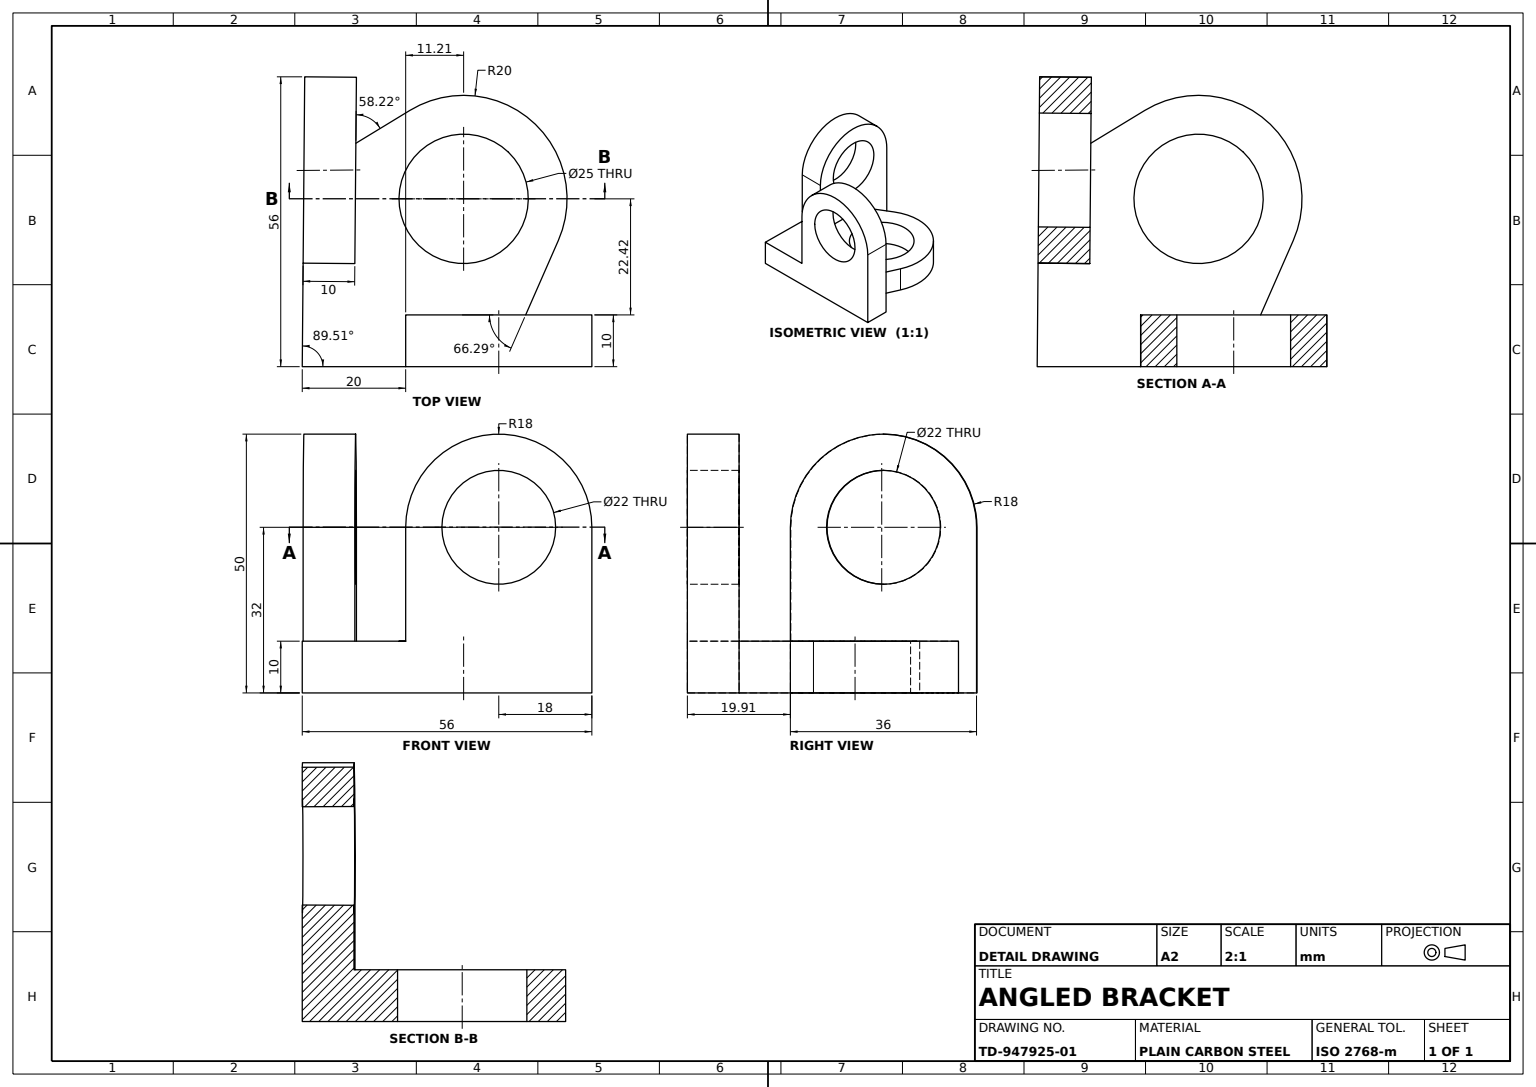
from build123d import *

# Parameters (mm, degrees)
BASE_PLATE_SKETCH_R = 12.5
BASE_PLATE_DEPTH    = 10
LUG_1_SKETCH_R      = 11
LUG_1_DEPTH         = 10
LUG_2_SKETCH_R      = 11
LUG_2_DEPTH         = 10


with BuildPart() as part:
    # Base Plate Sketch → Base Plate (new body)
    with BuildSketch(Plane(origin=(0, 0, 0), x_dir=(1, 0, 0), z_dir=(0, 1, 0))):
        with BuildLine():
            Line((-19.336184956, -21.171904289), (-25.4662576, -44.368099172))
            Line((-25.4662576, -44.368099172), (0, -71.281889743))
            Line((0, -71.281889743), (27.963619281, -44.368099172))
            Line((27.963619281, -44.368099172), (18.770242682, -19.376964714))
            ThreePointArc((18.770242682, -19.376964714), (-0.941023212, -6.304040126), (-19.336184956, -21.171904289))
        make_face()
        with Locations(Location((0, -26.281889743, 0), (0, 0, 270))):
            Circle(BASE_PLATE_SKETCH_R, mode=Mode.SUBTRACT)
    extrude(amount=BASE_PLATE_DEPTH)

    # Lug 1 Sketch → Lug 1 (add)
    with BuildSketch(Plane(origin=(35.61486713, 0, 37.004099536), x_dir=(0.720502211038311, 0, -0.6934526399754386), z_dir=(0.6934526399754386, 0, 0.720502211038311))):
        with BuildLine():
            Line((-29.430614625, 10), (-29.430614625, 32))
            ThreePointArc((-29.430614625, 32), (-11.430614625, 50), (6.569385375, 32))
            Line((6.569385375, 32), (6.569385375, 10))
            Line((6.569385375, 10), (6.569385375, 0))
            Line((6.569385375, 0), (-29.430614625, 0))
            Line((-29.430614625, 0), (-29.430614625, 10))
        make_face()
        with Locations((-11.430614625, 32)):
            Circle(LUG_1_SKETCH_R, mode=Mode.SUBTRACT)
    extrude(amount=-LUG_1_DEPTH)

    # Lug 2 Sketch → Lug 2 (add)
    with BuildSketch(Plane(origin=(-35.586548141, 0, 33.672559042), x_dir=(0.6873033475884168, 0, 0.7263705035267854), z_dir=(-0.7263705035267854, 0, 0.6873033475884168))):
        with BuildLine():
            Line((31.777062145, 32), (31.777062145, 0))
            Line((31.777062145, 0), (-4.222937855, 0))
            Line((-4.222937855, 0), (-4.222937855, 32))
            ThreePointArc((-4.222937855, 32), (13.777062145, 50), (31.777062145, 32))
        make_face()
        with Locations((13.777062145, 32)):
            Circle(LUG_2_SKETCH_R, mode=Mode.SUBTRACT)
    extrude(amount=-LUG_2_DEPTH)


solid = part.part
